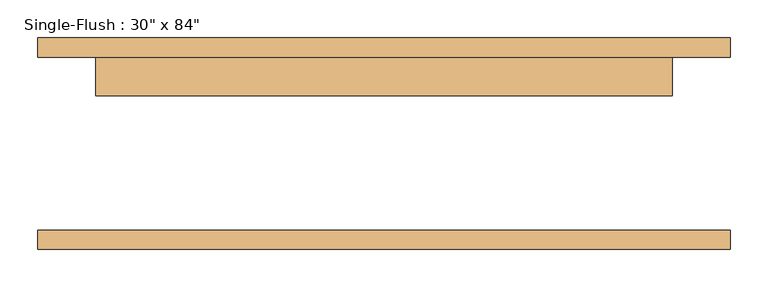
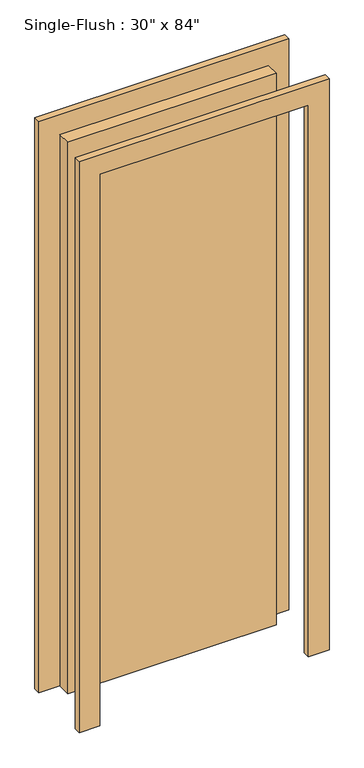
"""IFC4 building model written with IfcOpenShell, lengths in millimetres: door geometry."""

from ifc_helpers import new_model, si_unit, frame, origin, origin_with_axes, place, context, project, spatial, polyline, outline, extrude, source, transform, mapped, element, save


def door_bb98abfd(model_context):
    return source(origin(), model_context, "Body", "SweptSolid", [
        extrude(outline(polyline([(2209.8, -457.2), (0.0, -457.2), (0.0, -381.0), (2133.6, -381.0), (2133.6, 381.0), (0.0, 381.0), (0.0, 457.2), (2209.8, 457.2), (2209.8, -457.2)])), frame((0.0, 114.3, 0.0), z_axis=(0.0, 1.0, 0.0), x_axis=(0.0, 0.0, 1.0)), (0.0, 0.0, 1.0), 25.4),
        extrude(outline(polyline([(2209.8, 457.2), (2209.8, -457.2), (0.0, -457.2), (0.0, -381.0), (2133.6, -381.0), (2133.6, 381.0), (0.0, 381.0), (0.0, 457.2), (2209.8, 457.2)])), frame((0.0, -139.7, 0.0), z_axis=(0.0, 1.0, 0.0), x_axis=(0.0, 0.0, 1.0)), (0.0, 0.0, 1.0), 25.4),
        extrude(outline(polyline([(381.0, 63.5), (-381.0, 63.5), (-381.0, 114.3), (381.0, 114.3), (381.0, 63.5)])), origin_with_axes(), (0.0, 0.0, 1.0), 2133.6),
    ])


if __name__ == "__main__":
    model = new_model("IFC4")
    model_context = context("Model", 3, world=origin())
    ifc_project = project(units=[si_unit("LENGTHUNIT", "METRE", prefix="MILLI")], contexts=[model_context])
    site = spatial("IfcSite", under=ifc_project)
    building = spatial("IfcBuilding", under=site)
    placement = place(None, origin())
    door_shape = door_bb98abfd(model_context)
    element("IfcDoor", 1, ObjectType="Single-Flush : 30\" x 84\"", at=placement, inside=building, context=model_context, shape_type="MappedRepresentation", body=[
        mapped(door_shape, transform((0.0, 0.0, 0.0), x_axis=(1.0, 0.0, 0.0), y_axis=(0.0, 1.0, 0.0), z_axis=(0.0, 0.0, 1.0))),
    ])
    save(model, "model.ifc")

# Revit data of these elements
# Type "Single-Flush : 30\" x 84\""
#   Type Mark = "4"
#   Construction Type Id = "MDOOR"
#   Assembly Code = "C1020"
#   Analytic Construction = "Metal"
#   Thickness = 0' - 2"
#   Heat Transfer Coefficient (U) = 0.651978 BTU/(h·ft²·°F)
#   Height = 7' - 0"
#   Trim Projection Ext = 0' - 1"
#   Trim Projection Int = 0' - 1"
#   Trim Width = 0' - 3"
#   Width = 2' - 6"
#   Define Thermal Properties by = 1
#   Define Thermal Properties by = 1
#   Door Material = Door - Panel
#   Frame Material = Door - Frame
#   Visual Light Transmittance = 0
#   Solar Heat Gain Coefficient = 0
#   Function = (empty or 0)
#   Wall Closure = (empty or 0)
# Element 1 (IfcDoor, "Single-Flush : 30\" x 84\"")
#   Materials on its faces: "Door - Frame", "Door - Panel"
# Materials
#   "Door - Panel": class "Wood", colour RGB 210 159 95, transparency 0, Cost = 0
#   "Door - Frame": colour RGB 118 70 51, transparency 0, Cost = 0
